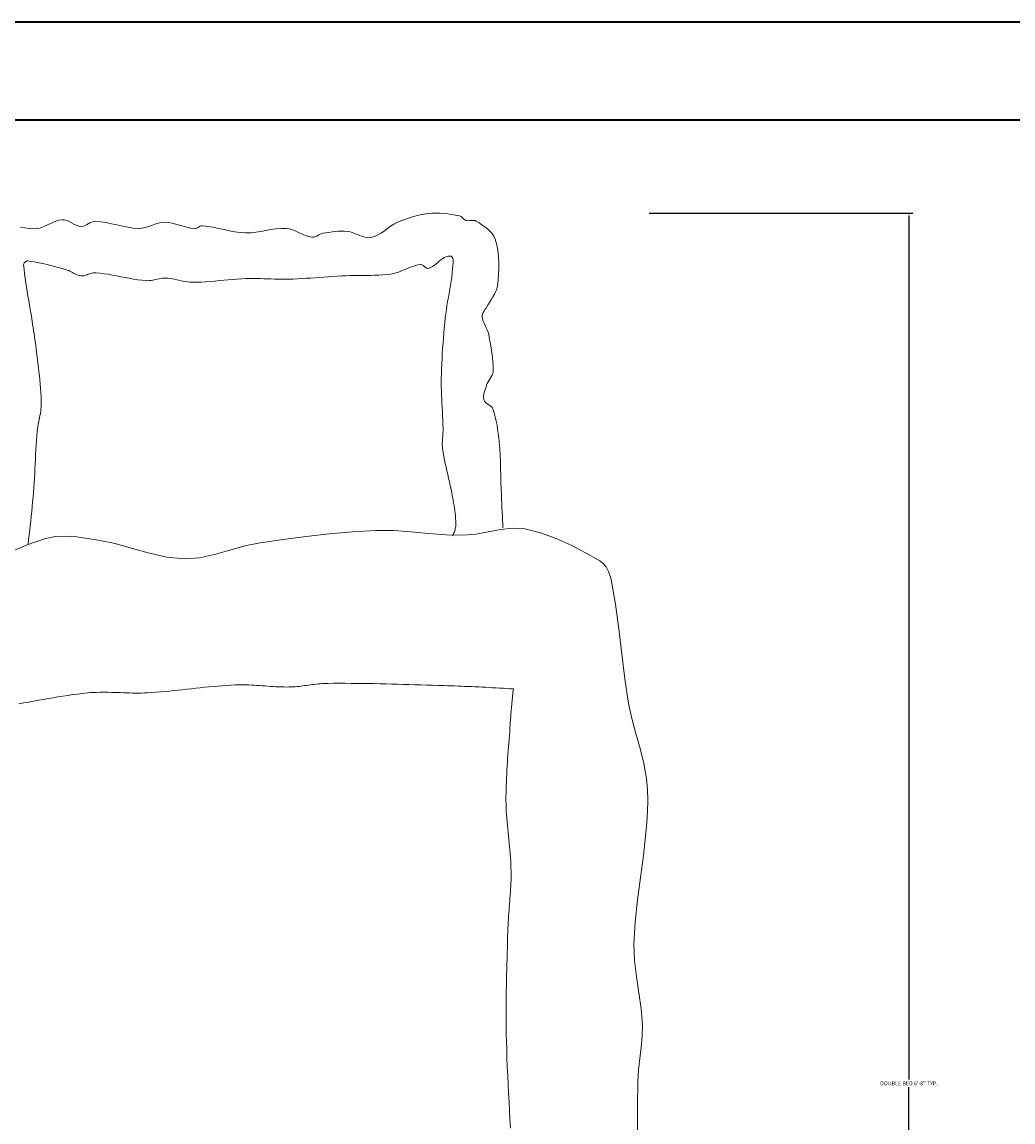
# Model space of a CAD drawing. Units: inches. Extents: x -36302355 to 648, y -221479757 to 75.
# Tile 27 of 37: x 220 to 265, y -218 to -167. Entities that reach past the tile are written whole.
import ezdxf

# ---------------------------------------------------------------- set-up
doc = ezdxf.new("R2010")
doc.units = ezdxf.units.IN
doc.header["$MEASUREMENT"] = 0
for name, color, linetype, lineweight in [('A-ANNO-DIMS', 2, 'Continuous', 18), ('A-FURN', 8, 'Continuous', 13), ('A-WALL', 7, 'Continuous', 35)]:
    doc.layers.add(name, color=color, linetype=linetype, lineweight=lineweight)
doc.styles.get("Standard").update_dxf_attribs({"font": 'arial.ttf'})
doc.dimstyles.get("Standard").update_dxf_attribs({"dimtxt": 0.18, "dimasz": 0.18, "dimexe": 0.18, "dimexo": 0.0625, "dimgap": 0.09, "dimtad": 0, "dimtih": 1, "dimtoh": 1, "dimdec": 0, "dimzin": 0, "dimdsep": 46, "dimlunit": 3, "dimtxsty": 'Standard', "dimcen": 0.09, "dimadec": 0, "dimazin": 0, "dimtfac": 1, "dimtdec": 0, "dimtofl": 0, "dimtmove": 0, "dimatfit": 3, "dimfxl": 1, "dimtolj": 1, "dimtzin": 0, "dimarcsym": 0})

# ---------------------------------------------------------------- blocks, each defined once
blk = doc.blocks.new('BED-DOUBLE')
for p, q in [((45.912, 79.943), (45.733, 79.9)), ((46.094, 79.977), (45.912, 79.943)), ((46.276, 80.001), (46.094, 79.977)), ((46.457, 80.015), (46.276, 80.001)), ((46.638, 80.019), (46.457, 80.015)), ((46.819, 80.013), (46.638, 80.019)), ((47.001, 80.001), (46.819, 80.013)), ((47.182, 79.981), (47.001, 80.001)), ((47.363, 79.957), (47.182, 79.981)), ((47.542, 79.928), (47.363, 79.957)), ((47.721, 79.897), (47.542, 79.928)), ((28.75, 79.461), (28.614, 79.399)), ((28.885, 79.529), (28.75, 79.461)), ((29.019, 79.595), (28.885, 79.529)), ((29.156, 79.653), (29.019, 79.595)), ((29.295, 79.695), (29.156, 79.653)), ((29.439, 79.716), (29.295, 79.695)), ((29.555, 79.707), (29.439, 79.716)), ((29.667, 79.676), (29.555, 79.707)), ((29.776, 79.63), (29.667, 79.676)), ((29.885, 79.575), (29.776, 79.63)), ((29.994, 79.518), (29.885, 79.575)), ((30.103, 79.467), (29.994, 79.518)), ((30.215, 79.429), (30.103, 79.467)), ((30.331, 79.412), (30.215, 79.429)), ((30.415, 79.419), (30.331, 79.412)), ((30.496, 79.445), (30.415, 79.419)), ((30.575, 79.483), (30.496, 79.445)), ((30.654, 79.527), (30.575, 79.483)), ((30.732, 79.571), (30.654, 79.527)), ((30.811, 79.61), (30.732, 79.571)), ((30.892, 79.636), (30.811, 79.61)), ((30.976, 79.644), (30.892, 79.636)), ((31.228, 79.624), (30.976, 79.644)), ((31.477, 79.585), (31.228, 79.624)), ((31.725, 79.534), (31.477, 79.585)), ((31.973, 79.478), (31.725, 79.534)), ((32.221, 79.421), (31.973, 79.478)), ((32.469, 79.372), (32.221, 79.421)), ((33.423, 79.406), (33.273, 79.362)), ((33.571, 79.458), (33.423, 79.406)), ((33.72, 79.51), (33.571, 79.458)), ((33.869, 79.555), (33.72, 79.51)), ((34.02, 79.587), (33.869, 79.555)), ((34.173, 79.598), (34.02, 79.587)), ((34.345, 79.587), (34.173, 79.598)), ((34.515, 79.557), (34.345, 79.587)), ((34.684, 79.516), (34.515, 79.557)), ((34.852, 79.467), (34.684, 79.516)), ((35.02, 79.416), (34.852, 79.467)), ((35.188, 79.369), (35.02, 79.416)), ((35.804, 79.42), (35.758, 79.398)), ((35.85, 79.435), (35.804, 79.42)), ((35.898, 79.439), (35.85, 79.435)), ((36.149, 79.41), (35.898, 79.439)), ((36.398, 79.368), (36.149, 79.41)), ((44.554, 79.421), (44.409, 79.317)), ((44.703, 79.516), (44.554, 79.421)), ((44.859, 79.595), (44.703, 79.516)), ((45.03, 79.665), (44.859, 79.595)), ((45.203, 79.731), (45.03, 79.665)), ((45.378, 79.793), (45.203, 79.731)), ((45.554, 79.85), (45.378, 79.793)), ((45.733, 79.9), (45.554, 79.85)), ((47.762, 79.883), (47.721, 79.897)), ((47.799, 79.86), (47.762, 79.883)), ((47.832, 79.831), (47.799, 79.86)), ((47.865, 79.797), (47.832, 79.831)), ((47.897, 79.763), (47.865, 79.797)), ((47.93, 79.732), (47.897, 79.763)), ((47.966, 79.705), (47.93, 79.732)), ((48.005, 79.687), (47.966, 79.705)), ((48.065, 79.675), (48.005, 79.687)), ((48.126, 79.673), (48.065, 79.675)), ((48.189, 79.677), (48.126, 79.673)), ((48.253, 79.684), (48.189, 79.677)), ((48.316, 79.688), (48.253, 79.684)), ((48.376, 79.687), (48.316, 79.688)), ((48.434, 79.676), (48.376, 79.687)), ((48.487, 79.652), (48.434, 79.676)), ((48.617, 79.57), (48.487, 79.652)), ((48.749, 79.484), (48.617, 79.57)), ((48.879, 79.394), (48.749, 79.484)), ((27.733, 79.348), (27.532, 79.381)), ((27.935, 79.319), (27.733, 79.348)), ((28.135, 79.305), (27.935, 79.319)), ((28.332, 79.316), (28.135, 79.305)), ((28.475, 79.348), (28.332, 79.316)), ((28.614, 79.399), (28.475, 79.348)), ((32.718, 79.336), (32.469, 79.372)), ((32.97, 79.321), (32.718, 79.336)), ((33.123, 79.331), (32.97, 79.321)), ((33.273, 79.362), (33.123, 79.331)), ((35.358, 79.33), (35.188, 79.369)), ((35.529, 79.305), (35.358, 79.33)), ((35.577, 79.308), (35.529, 79.305)), ((35.623, 79.323), (35.577, 79.308)), ((35.669, 79.345), (35.623, 79.323)), ((35.714, 79.371), (35.669, 79.345)), ((35.758, 79.398), (35.714, 79.371)), ((36.646, 79.318), (36.398, 79.368)), ((36.894, 79.264), (36.646, 79.318)), ((37.142, 79.212), (36.894, 79.264)), ((37.39, 79.167), (37.142, 79.212)), ((37.64, 79.133), (37.39, 79.167)), ((37.891, 79.115), (37.64, 79.133)), ((38.124, 79.119), (37.891, 79.115)), ((38.357, 79.144), (38.124, 79.119)), ((38.588, 79.18), (38.357, 79.144)), ((38.82, 79.223), (38.588, 79.18)), ((39.051, 79.265), (38.82, 79.223)), ((39.283, 79.299), (39.051, 79.265)), ((39.515, 79.318), (39.283, 79.299)), ((39.748, 79.315), (39.515, 79.318)), ((39.902, 79.292), (39.748, 79.315)), ((40.051, 79.248), (39.902, 79.292)), ((40.198, 79.189), (40.051, 79.248)), ((40.343, 79.122), (40.198, 79.189)), ((40.488, 79.055), (40.343, 79.122)), ((40.634, 78.992), (40.488, 79.055)), ((40.783, 78.942), (40.634, 78.992)), ((40.936, 78.91), (40.783, 78.942)), ((41.002, 78.91), (40.936, 78.91)), ((41.066, 78.924), (41.002, 78.91)), ((41.128, 78.95), (41.066, 78.924)), ((41.19, 78.981), (41.128, 78.95)), ((41.252, 79.016), (41.19, 78.981)), ((41.315, 79.048), (41.252, 79.016)), ((41.378, 79.075), (41.315, 79.048)), ((41.444, 79.093), (41.378, 79.075)), ((41.582, 79.116), (41.444, 79.093)), ((41.721, 79.137), (41.582, 79.116)), ((41.86, 79.157), (41.721, 79.137)), ((42, 79.173), (41.86, 79.157)), ((42.139, 79.184), (42, 79.173)), ((42.279, 79.19), (42.139, 79.184)), ((42.419, 79.19), (42.279, 79.19)), ((42.558, 79.182), (42.419, 79.19)), ((42.698, 79.158), (42.558, 79.182)), ((42.835, 79.114), (42.698, 79.158)), ((42.971, 79.06), (42.835, 79.114)), ((43.106, 79.003), (42.971, 79.06)), ((43.241, 78.95), (43.106, 79.003)), ((43.377, 78.91), (43.241, 78.95)), ((43.513, 78.89), (43.377, 78.91)), ((43.817, 78.944), (43.651, 78.898)), ((43.972, 79.016), (43.817, 78.944)), ((44.121, 79.107), (43.972, 79.016)), ((44.266, 79.21), (44.121, 79.107)), ((44.409, 79.317), (44.266, 79.21)), ((49.004, 79.298), (48.879, 79.394)), ((49.119, 79.194), (49.004, 79.298)), ((49.219, 79.081), (49.119, 79.194)), ((49.301, 78.957), (49.219, 79.081)), ((49.36, 78.82), (49.301, 78.957)), ((43.651, 78.898), (43.513, 78.89)), ((49.432, 78.561), (49.36, 78.82)), ((49.482, 78.296), (49.432, 78.561)), ((46.868, 77.87), (46.947, 77.928)), ((46.947, 77.928), (47.028, 77.978)), ((47.028, 77.978), (47.112, 78.016)), ((47.112, 78.016), (47.2, 78.041)), ((47.2, 78.041), (47.293, 78.049)), ((47.293, 78.049), (47.337, 78.04)), ((47.337, 78.04), (47.371, 78.018)), ((47.371, 78.018), (47.396, 77.983)), ((47.396, 77.983), (47.413, 77.939)), ((47.413, 77.939), (47.423, 77.887)), ((49.513, 78.027), (49.482, 78.296)), ((49.527, 77.755), (49.513, 78.027)), ((27.683, 77.649), (27.684, 77.671)), ((27.699, 77.441), (27.683, 77.649)), ((27.684, 77.671), (27.689, 77.693)), ((27.689, 77.693), (27.699, 77.715)), ((27.699, 77.715), (27.712, 77.735)), ((27.721, 77.234), (27.699, 77.441)), ((27.712, 77.735), (27.728, 77.755)), ((27.728, 77.755), (27.746, 77.773)), ((27.746, 77.773), (27.767, 77.789)), ((27.767, 77.789), (27.789, 77.803)), ((27.789, 77.803), (27.812, 77.813)), ((27.812, 77.813), (27.835, 77.821)), ((27.835, 77.821), (27.858, 77.824)), ((27.858, 77.824), (27.88, 77.824)), ((27.88, 77.824), (28.029, 77.804)), ((28.029, 77.804), (28.178, 77.781)), ((28.178, 77.781), (28.326, 77.754)), ((28.326, 77.754), (28.474, 77.723)), ((28.474, 77.723), (28.621, 77.691)), ((28.621, 77.691), (28.768, 77.655)), ((28.768, 77.655), (28.915, 77.618)), ((28.915, 77.618), (29.061, 77.58)), ((29.061, 77.58), (29.206, 77.54)), ((29.206, 77.54), (29.352, 77.499)), ((29.352, 77.499), (29.497, 77.458)), ((29.497, 77.458), (29.643, 77.417)), ((29.643, 77.417), (29.7, 77.398)), ((29.7, 77.398), (29.757, 77.376)), ((45.023, 77.35), (45.135, 77.394)), ((45.135, 77.394), (45.245, 77.439)), ((45.245, 77.439), (45.356, 77.485)), ((45.356, 77.485), (45.467, 77.529)), ((45.467, 77.529), (45.579, 77.57)), ((45.579, 77.57), (45.692, 77.607)), ((45.692, 77.607), (45.806, 77.636)), ((45.806, 77.636), (45.922, 77.659)), ((45.922, 77.659), (45.956, 77.659)), ((45.956, 77.659), (45.988, 77.65)), ((45.988, 77.65), (46.02, 77.634)), ((46.02, 77.634), (46.051, 77.613)), ((46.051, 77.613), (46.082, 77.589)), ((46.082, 77.589), (46.112, 77.564)), ((46.112, 77.564), (46.142, 77.538)), ((46.142, 77.538), (46.172, 77.515)), ((46.172, 77.515), (46.203, 77.496)), ((46.203, 77.496), (46.234, 77.483)), ((46.234, 77.483), (46.266, 77.478)), ((46.266, 77.478), (46.299, 77.482)), ((46.299, 77.482), (46.388, 77.515)), ((46.388, 77.515), (46.473, 77.56)), ((46.473, 77.56), (46.555, 77.615)), ((46.555, 77.615), (46.635, 77.677)), ((46.635, 77.677), (46.713, 77.741)), ((46.713, 77.741), (46.79, 77.807)), ((46.79, 77.807), (46.868, 77.87)), ((47.4, 77.462), (47.383, 77.273)), ((47.405, 77.515), (47.4, 77.462)), ((47.412, 77.574), (47.405, 77.515)), ((47.418, 77.637), (47.412, 77.574)), ((47.424, 77.701), (47.418, 77.637)), ((47.423, 77.887), (47.427, 77.828)), ((47.427, 77.766), (47.424, 77.701)), ((47.427, 77.828), (47.427, 77.766)), ((49.513, 77.208), (49.526, 77.481)), ((49.526, 77.481), (49.527, 77.755)), ((27.746, 77.027), (27.721, 77.234)), ((27.776, 76.821), (27.746, 77.027)), ((29.757, 77.376), (29.813, 77.349)), ((29.813, 77.349), (29.867, 77.321)), ((29.867, 77.321), (29.922, 77.292)), ((29.922, 77.292), (29.977, 77.263)), ((29.977, 77.263), (30.031, 77.234)), ((30.031, 77.234), (30.086, 77.207)), ((30.086, 77.207), (30.142, 77.184)), ((30.142, 77.184), (30.199, 77.164)), ((30.199, 77.164), (30.257, 77.148)), ((30.257, 77.148), (30.316, 77.139)), ((30.316, 77.139), (30.374, 77.137)), ((30.374, 77.137), (30.43, 77.142)), ((30.43, 77.142), (30.487, 77.153)), ((30.487, 77.153), (30.543, 77.169)), ((30.543, 77.169), (30.599, 77.187)), ((30.599, 77.187), (30.656, 77.207)), ((30.656, 77.207), (30.712, 77.227)), ((30.712, 77.227), (30.768, 77.246)), ((30.768, 77.246), (30.824, 77.261)), ((30.824, 77.261), (30.881, 77.273)), ((30.881, 77.273), (30.938, 77.28)), ((30.938, 77.28), (30.995, 77.28)), ((30.995, 77.28), (31.19, 77.261)), ((31.19, 77.261), (31.384, 77.237)), ((31.384, 77.237), (31.577, 77.207)), ((31.577, 77.207), (31.77, 77.173)), ((31.77, 77.173), (31.963, 77.137)), ((31.963, 77.137), (32.155, 77.099)), ((32.155, 77.099), (32.348, 77.062)), ((32.348, 77.062), (32.54, 77.025)), ((32.54, 77.025), (32.733, 76.991)), ((32.733, 76.991), (32.927, 76.961)), ((32.927, 76.961), (33.12, 76.936)), ((33.12, 76.936), (33.315, 76.917)), ((33.315, 76.917), (33.39, 76.915)), ((33.39, 76.915), (33.465, 76.919)), ((33.465, 76.919), (33.54, 76.927)), ((33.54, 76.927), (33.614, 76.939)), ((33.614, 76.939), (33.689, 76.954)), ((33.689, 76.954), (33.763, 76.97)), ((33.763, 76.97), (33.838, 76.986)), ((33.838, 76.986), (33.912, 77.002)), ((33.912, 77.002), (33.987, 77.015)), ((33.987, 77.015), (34.062, 77.026)), ((34.062, 77.026), (34.137, 77.032)), ((34.137, 77.032), (34.212, 77.032)), ((34.212, 77.032), (34.314, 77.026)), ((34.314, 77.026), (34.416, 77.014)), ((34.416, 77.014), (34.517, 76.997)), ((34.517, 76.997), (34.618, 76.978)), ((34.618, 76.978), (34.718, 76.956)), ((34.718, 76.956), (34.819, 76.934)), ((34.819, 76.934), (34.92, 76.912)), ((34.92, 76.912), (35.02, 76.891)), ((35.02, 76.891), (35.121, 76.873)), ((36.05, 76.866), (36.258, 76.881)), ((36.258, 76.881), (36.465, 76.899)), ((36.465, 76.899), (36.673, 76.918)), ((36.673, 76.918), (36.88, 76.938)), ((36.88, 76.938), (37.088, 76.957)), ((37.088, 76.957), (37.296, 76.976)), ((37.296, 76.976), (37.503, 76.992)), ((37.503, 76.992), (37.711, 77.005)), ((37.711, 77.005), (37.919, 77.014)), ((37.919, 77.014), (38.081, 77.017)), ((38.081, 77.017), (38.242, 77.017)), ((38.242, 77.017), (38.404, 77.015)), ((38.404, 77.015), (38.566, 77.011)), ((38.566, 77.011), (38.727, 77.006)), ((38.727, 77.006), (38.889, 77)), ((38.889, 77), (39.051, 76.993)), ((39.051, 76.993), (39.212, 76.988)), ((39.212, 76.988), (39.374, 76.984)), ((39.374, 76.984), (39.536, 76.981)), ((39.536, 76.981), (39.697, 76.981)), ((39.697, 76.981), (39.859, 76.984)), ((39.859, 76.984), (40.063, 76.991)), ((40.063, 76.991), (40.267, 77)), ((40.267, 77), (40.471, 77.011)), ((40.471, 77.011), (40.675, 77.024)), ((40.675, 77.024), (40.879, 77.038)), ((40.879, 77.038), (41.082, 77.053)), ((41.082, 77.053), (41.286, 77.068)), ((41.286, 77.068), (41.49, 77.083)), ((41.49, 77.083), (41.694, 77.098)), ((41.694, 77.098), (41.898, 77.112)), ((41.898, 77.112), (42.102, 77.125)), ((42.102, 77.125), (42.306, 77.136)), ((42.306, 77.136), (42.494, 77.144)), ((42.494, 77.144), (42.683, 77.148)), ((42.683, 77.148), (42.872, 77.151)), ((42.872, 77.151), (43.061, 77.152)), ((43.061, 77.152), (43.25, 77.152)), ((43.25, 77.152), (43.439, 77.153)), ((43.439, 77.153), (43.628, 77.156)), ((43.628, 77.156), (43.817, 77.161)), ((43.817, 77.161), (44.005, 77.169)), ((44.005, 77.169), (44.193, 77.181)), ((44.193, 77.181), (44.381, 77.199)), ((44.381, 77.199), (44.568, 77.222)), ((44.568, 77.222), (44.684, 77.244)), ((44.684, 77.244), (44.799, 77.273)), ((44.799, 77.273), (44.912, 77.309)), ((44.912, 77.309), (45.023, 77.35)), ((47.334, 76.896), (47.305, 76.708)), ((47.36, 77.084), (47.334, 76.896)), ((47.383, 77.273), (47.36, 77.084)), ((49.459, 76.667), (49.49, 76.936)), ((49.49, 76.936), (49.513, 77.208)), ((27.808, 76.615), (27.776, 76.821)), ((27.843, 76.41), (27.808, 76.615)), ((27.879, 76.204), (27.843, 76.41)), ((35.121, 76.873), (35.223, 76.858)), ((35.223, 76.858), (35.324, 76.848)), ((35.324, 76.848), (35.426, 76.845)), ((35.426, 76.845), (35.634, 76.847)), ((35.634, 76.847), (35.842, 76.854)), ((35.842, 76.854), (36.05, 76.866)), ((47.273, 76.52), (47.241, 76.333)), ((47.305, 76.708), (47.273, 76.52)), ((49.327, 76.292), (49.387, 76.412)), ((49.387, 76.412), (49.432, 76.537)), ((49.432, 76.537), (49.459, 76.667)), ((27.915, 75.999), (27.879, 76.204)), ((27.952, 75.793), (27.915, 75.999)), ((47.175, 75.958), (47.144, 75.77)), ((47.208, 76.145), (47.175, 75.958)), ((47.241, 76.333), (47.208, 76.145)), ((49.036, 75.827), (49.108, 75.944)), ((49.108, 75.944), (49.184, 76.059)), ((49.184, 76.059), (49.258, 76.175)), ((49.258, 76.175), (49.327, 76.292)), ((27.987, 75.588), (27.952, 75.793)), ((28.021, 75.382), (27.987, 75.588)), ((28.053, 75.176), (28.021, 75.382)), ((47.089, 75.394), (47.068, 75.205)), ((47.115, 75.582), (47.089, 75.394)), ((47.144, 75.77), (47.115, 75.582)), ((48.767, 75.329), (48.782, 75.386)), ((48.782, 75.386), (48.806, 75.441)), ((48.806, 75.441), (48.836, 75.495)), ((48.836, 75.495), (48.871, 75.549)), ((48.871, 75.549), (48.907, 75.602)), ((48.907, 75.602), (48.941, 75.655)), ((48.941, 75.655), (48.971, 75.709)), ((48.971, 75.709), (49.036, 75.827)), ((28.074, 75.036), (28.053, 75.176)), ((28.095, 74.896), (28.074, 75.036)), ((28.117, 74.755), (28.095, 74.896)), ((47.044, 74.972), (47.022, 74.739)), ((47.068, 75.205), (47.044, 74.972)), ((48.764, 75.269), (48.767, 75.329)), ((48.781, 75.161), (48.764, 75.269)), ((48.812, 75.056), (48.781, 75.161)), ((48.854, 74.954), (48.812, 75.056)), ((48.901, 74.853), (48.854, 74.954)), ((28.139, 74.615), (28.117, 74.755)), ((28.161, 74.475), (28.139, 74.615)), ((28.182, 74.335), (28.161, 74.475)), ((47.001, 74.505), (46.981, 74.272)), ((47.022, 74.739), (47.001, 74.505)), ((48.95, 74.751), (48.901, 74.853)), ((48.996, 74.649), (48.95, 74.751)), ((49.036, 74.546), (48.996, 74.649)), ((49.064, 74.439), (49.036, 74.546)), ((49.105, 74.229), (49.064, 74.439)), ((28.203, 74.194), (28.182, 74.335)), ((28.224, 74.054), (28.203, 74.194)), ((28.243, 73.914), (28.224, 74.054)), ((28.262, 73.773), (28.243, 73.914)), ((46.962, 74.038), (46.945, 73.805)), ((46.981, 74.272), (46.962, 74.038)), ((49.144, 74.017), (49.105, 74.229)), ((49.181, 73.805), (49.144, 74.017)), ((28.279, 73.632), (28.262, 73.773)), ((28.296, 73.491), (28.279, 73.632)), ((28.317, 73.302), (28.296, 73.491)), ((46.929, 73.571), (46.916, 73.337)), ((46.945, 73.805), (46.929, 73.571)), ((49.212, 73.592), (49.181, 73.805)), ((49.238, 73.379), (49.212, 73.592)), ((49.255, 73.166), (49.238, 73.379)), ((28.339, 73.113), (28.317, 73.302)), ((28.361, 72.924), (28.339, 73.113)), ((28.383, 72.734), (28.361, 72.924)), ((46.894, 72.869), (46.886, 72.635)), ((46.904, 73.103), (46.894, 72.869)), ((46.916, 73.337), (46.904, 73.103)), ((49.263, 72.952), (49.255, 73.166)), ((49.26, 72.738), (49.263, 72.952)), ((28.404, 72.545), (28.383, 72.734)), ((28.424, 72.356), (28.404, 72.545)), ((28.442, 72.166), (28.424, 72.356)), ((46.88, 72.401), (46.878, 72.212)), ((46.886, 72.635), (46.88, 72.401)), ((49.04, 72.269), (49.087, 72.345)), ((49.087, 72.345), (49.136, 72.42)), ((49.136, 72.42), (49.181, 72.496)), ((49.181, 72.496), (49.22, 72.573)), ((49.22, 72.573), (49.248, 72.654)), ((49.248, 72.654), (49.26, 72.738)), ((28.458, 71.976), (28.442, 72.166)), ((28.471, 71.786), (28.458, 71.976)), ((46.878, 72.212), (46.88, 72.024)), ((46.88, 72.024), (46.885, 71.835)), ((46.885, 71.835), (46.892, 71.647)), ((48.856, 71.777), (48.88, 71.861)), ((48.88, 71.861), (48.909, 71.945)), ((48.909, 71.945), (48.938, 72.028)), ((48.938, 72.028), (48.965, 72.11)), ((48.965, 72.11), (48.998, 72.191)), ((48.998, 72.191), (49.04, 72.269)), ((28.482, 71.596), (28.471, 71.786)), ((28.488, 71.406), (28.482, 71.596)), ((28.491, 71.216), (28.488, 71.406)), ((46.892, 71.647), (46.902, 71.458)), ((46.902, 71.458), (46.912, 71.27)), ((48.827, 71.607), (48.837, 71.692)), ((48.828, 71.523), (48.827, 71.607)), ((48.842, 71.44), (48.828, 71.523)), ((48.837, 71.692), (48.856, 71.777)), ((48.872, 71.375), (48.842, 71.44)), ((48.919, 71.32), (48.872, 71.375)), ((48.978, 71.271), (48.919, 71.32)), ((28.432, 70.709), (28.451, 70.81)), ((28.451, 70.81), (28.467, 70.911)), ((28.467, 70.911), (28.48, 71.012)), ((28.48, 71.012), (28.488, 71.114)), ((28.488, 71.114), (28.491, 71.216)), ((46.912, 71.27), (46.923, 71.081)), ((46.923, 71.081), (46.934, 70.893)), ((46.934, 70.893), (46.944, 70.704)), ((49.043, 71.226), (48.978, 71.271)), ((49.109, 71.182), (49.043, 71.226)), ((49.17, 71.134), (49.109, 71.182)), ((49.221, 71.08), (49.17, 71.134)), ((49.256, 71.016), (49.221, 71.08)), ((49.316, 70.833), (49.256, 71.016)), ((49.367, 70.648), (49.316, 70.833)), ((28.33, 70.205), (28.348, 70.306)), ((28.348, 70.306), (28.368, 70.407)), ((28.368, 70.407), (28.389, 70.508)), ((28.389, 70.508), (28.411, 70.608)), ((28.411, 70.608), (28.432, 70.709)), ((46.944, 70.704), (46.954, 70.516)), ((46.954, 70.516), (46.961, 70.327)), ((46.961, 70.327), (46.966, 70.138)), ((49.409, 70.46), (49.367, 70.648)), ((49.445, 70.27), (49.409, 70.46)), ((28.285, 69.785), (28.303, 70.002)), ((28.303, 70.002), (28.315, 70.104)), ((28.315, 70.104), (28.33, 70.205)), ((46.954, 69.822), (46.947, 69.743)), ((46.959, 69.901), (46.954, 69.822)), ((46.964, 69.98), (46.959, 69.901)), ((46.966, 70.059), (46.964, 69.98)), ((46.966, 70.138), (46.966, 70.059)), ((49.474, 70.079), (49.445, 70.27)), ((49.499, 69.887), (49.474, 70.079)), ((49.521, 69.695), (49.499, 69.887)), ((28.244, 69.133), (28.256, 69.35)), ((28.256, 69.35), (28.27, 69.568)), ((28.27, 69.568), (28.285, 69.785)), ((46.932, 69.506), (46.93, 69.427)), ((46.93, 69.427), (46.93, 69.349)), ((46.93, 69.349), (46.934, 69.27)), ((46.936, 69.585), (46.932, 69.506)), ((46.941, 69.664), (46.936, 69.585)), ((46.947, 69.743), (46.941, 69.664)), ((49.541, 69.503), (49.521, 69.695)), ((49.567, 69.196), (49.541, 69.503)), ((28.223, 68.697), (28.234, 68.915)), ((28.234, 68.915), (28.244, 69.133)), ((46.934, 69.27), (46.943, 69.192)), ((46.943, 69.192), (46.968, 69.02)), ((46.968, 69.02), (46.997, 68.85)), ((46.997, 68.85), (47.03, 68.679)), ((49.586, 68.889), (49.567, 69.196)), ((49.6, 68.581), (49.586, 68.889)), ((28.203, 68.262), (28.213, 68.48)), ((28.213, 68.48), (28.223, 68.697)), ((47.03, 68.679), (47.066, 68.51)), ((47.066, 68.51), (47.103, 68.34)), ((47.103, 68.34), (47.142, 68.171)), ((49.611, 68.273), (49.6, 68.581)), ((28.166, 67.61), (28.18, 67.827)), ((28.18, 67.827), (28.192, 68.045)), ((28.192, 68.045), (28.203, 68.262)), ((47.142, 68.171), (47.182, 68.002)), ((47.182, 68.002), (47.221, 67.833)), ((47.221, 67.833), (47.26, 67.664)), ((49.619, 67.964), (49.611, 68.273)), ((49.627, 67.656), (49.619, 67.964)), ((28.132, 67.176), (28.15, 67.392)), ((28.15, 67.392), (28.166, 67.61)), ((47.26, 67.664), (47.297, 67.495)), ((47.297, 67.495), (47.332, 67.325)), ((47.332, 67.325), (47.364, 67.155)), ((49.636, 67.348), (49.627, 67.656)), ((49.647, 67.04), (49.636, 67.348)), ((28.094, 66.742), (28.113, 66.959)), ((28.113, 66.959), (28.132, 67.176)), ((47.364, 67.155), (47.385, 67.039)), ((47.385, 67.039), (47.406, 66.924)), ((47.406, 66.924), (47.428, 66.809)), ((47.428, 66.809), (47.448, 66.693)), ((49.655, 66.854), (49.647, 67.04)), ((49.664, 66.668), (49.655, 66.854)), ((28.032, 66.093), (28.053, 66.309)), ((28.053, 66.309), (28.074, 66.526)), ((28.074, 66.526), (28.094, 66.742)), ((47.448, 66.693), (47.468, 66.577)), ((47.468, 66.577), (47.487, 66.462)), ((47.487, 66.462), (47.504, 66.346)), ((47.504, 66.346), (47.519, 66.23)), ((49.672, 66.482), (49.664, 66.668)), ((49.68, 66.296), (49.672, 66.482)), ((49.689, 66.11), (49.68, 66.296)), ((27.987, 65.66), (28.01, 65.876)), ((28.01, 65.876), (28.032, 66.093)), ((47.519, 66.23), (47.532, 66.113)), ((47.532, 66.113), (47.543, 65.997)), ((47.543, 65.997), (47.55, 65.88)), ((47.55, 65.88), (47.554, 65.763)), ((47.554, 65.763), (47.553, 65.713)), ((49.697, 65.924), (49.689, 66.11)), ((49.706, 65.738), (49.697, 65.924)), ((27.938, 65.228), (27.963, 65.444)), ((27.963, 65.444), (27.987, 65.66)), ((41.735, 65.273), (40.671, 65.153)), ((42.802, 65.366), (41.735, 65.273)), ((43.87, 65.425), (42.802, 65.366)), ((44.678, 65.422), (43.87, 65.425)), ((45.485, 65.369), (44.678, 65.422)), ((46.292, 65.296), (45.485, 65.369)), ((47.1, 65.235), (46.292, 65.296)), ((47.445, 65.274), (47.422, 65.229)), ((47.466, 65.32), (47.445, 65.274)), ((47.484, 65.367), (47.466, 65.32)), ((47.501, 65.415), (47.484, 65.367)), ((47.515, 65.464), (47.501, 65.415)), ((47.527, 65.513), (47.515, 65.464)), ((47.537, 65.563), (47.527, 65.513)), ((47.545, 65.613), (47.537, 65.563)), ((47.55, 65.663), (47.545, 65.613)), ((47.553, 65.713), (47.55, 65.663)), ((48.474, 65.264), (47.908, 65.214)), ((49.04, 65.369), (48.474, 65.264)), ((49.604, 65.477), (49.04, 65.369)), ((50.166, 65.538), (49.604, 65.477)), ((49.715, 65.552), (49.706, 65.738)), ((50.724, 65.499), (50.166, 65.538)), ((51.45, 65.318), (50.724, 65.499)), ((52.158, 65.065), (51.45, 65.318)), ((27.839, 64.768), (27.022, 64.416)), ((28.68, 65.056), (27.839, 64.768)), ((27.887, 64.796), (27.913, 65.012)), ((27.913, 65.012), (27.938, 65.228)), ((29.152, 65.148), (28.68, 65.056)), ((29.636, 65.165), (29.152, 65.148)), ((30.126, 65.13), (29.636, 65.165)), ((30.616, 65.064), (30.126, 65.13)), ((31.101, 64.99), (30.616, 65.064)), ((31.896, 64.828), (31.101, 64.99)), ((32.683, 64.608), (31.896, 64.828)), ((38.549, 64.862), (37.849, 64.716)), ((39.609, 65.014), (38.549, 64.862)), ((40.671, 65.153), (39.609, 65.014)), ((47.908, 65.214), (47.1, 65.235)), ((47.422, 65.229), (47.397, 65.186)), ((52.846, 64.755), (52.158, 65.065)), ((53.517, 64.405), (52.846, 64.755)), ((33.469, 64.384), (32.683, 64.608)), ((34.259, 64.206), (33.469, 64.384)), ((36.463, 64.326), (35.767, 64.177)), ((37.155, 64.522), (36.463, 64.326)), ((37.849, 64.716), (37.155, 64.522)), ((54.172, 64.032), (53.517, 64.405)), ((35.061, 64.125), (34.259, 64.206)), ((35.767, 64.177), (35.061, 64.125)), ((54.33, 63.91), (54.172, 64.032)), ((54.459, 63.752), (54.33, 63.91)), ((54.561, 63.57), (54.459, 63.752)), ((54.638, 63.375), (54.561, 63.57)), ((54.689, 63.176), (54.638, 63.375)), ((54.886, 62.042), (54.689, 63.176)), ((55.039, 60.9), (54.886, 62.042)), ((55.175, 59.755), (55.039, 60.9)), ((55.318, 58.611), (55.175, 59.755)), ((35.594, 58.175), (35.393, 58.153)), ((35.796, 58.197), (35.594, 58.175)), ((35.998, 58.218), (35.796, 58.197)), ((36.2, 58.239), (35.998, 58.218)), ((36.401, 58.258), (36.2, 58.239)), ((36.603, 58.276), (36.401, 58.258)), ((36.806, 58.292), (36.603, 58.276)), ((37.008, 58.306), (36.806, 58.292)), ((37.21, 58.318), (37.008, 58.306)), ((37.413, 58.327), (37.21, 58.318)), ((37.537, 58.331), (37.413, 58.327)), ((37.661, 58.333), (37.537, 58.331)), ((37.785, 58.332), (37.661, 58.333)), ((37.909, 58.329), (37.785, 58.332)), ((38.034, 58.325), (37.909, 58.329)), ((38.158, 58.319), (38.034, 58.325)), ((38.282, 58.313), (38.158, 58.319)), ((38.406, 58.305), (38.282, 58.313)), ((38.53, 58.296), (38.406, 58.305)), ((38.654, 58.288), (38.53, 58.296)), ((38.779, 58.279), (38.654, 58.288)), ((38.903, 58.27), (38.779, 58.279)), ((39.027, 58.261), (38.903, 58.27)), ((39.151, 58.253), (39.027, 58.261)), ((39.275, 58.246), (39.151, 58.253)), ((39.4, 58.241), (39.275, 58.246)), ((39.524, 58.236), (39.4, 58.241)), ((39.648, 58.233), (39.524, 58.236)), ((39.772, 58.232), (39.648, 58.233)), ((39.896, 58.233), (39.772, 58.232)), ((39.985, 58.235), (39.896, 58.233)), ((40.073, 58.24), (39.985, 58.235)), ((40.162, 58.246), (40.073, 58.24)), ((40.25, 58.254), (40.162, 58.246)), ((40.338, 58.262), (40.25, 58.254)), ((40.426, 58.272), (40.338, 58.262)), ((40.514, 58.283), (40.426, 58.272)), ((40.603, 58.294), (40.514, 58.283)), ((40.691, 58.306), (40.603, 58.294)), ((40.779, 58.318), (40.691, 58.306)), ((40.867, 58.33), (40.779, 58.318)), ((40.955, 58.342), (40.867, 58.33)), ((41.043, 58.353), (40.955, 58.342)), ((41.131, 58.363), (41.043, 58.353)), ((41.219, 58.373), (41.131, 58.363)), ((41.307, 58.381), (41.219, 58.373)), ((41.395, 58.389), (41.307, 58.381)), ((41.484, 58.394), (41.395, 58.389)), ((41.572, 58.398), (41.484, 58.394)), ((41.661, 58.4), (41.572, 58.398)), ((41.928, 58.402), (41.661, 58.4)), ((42.196, 58.402), (41.928, 58.402)), ((42.464, 58.402), (42.196, 58.402)), ((42.731, 58.401), (42.464, 58.402)), ((42.999, 58.398), (42.731, 58.401)), ((43.267, 58.395), (42.999, 58.398)), ((43.535, 58.391), (43.267, 58.395)), ((43.802, 58.386), (43.535, 58.391)), ((44.07, 58.381), (43.802, 58.386)), ((44.338, 58.375), (44.07, 58.381)), ((44.605, 58.368), (44.338, 58.375)), ((44.873, 58.362), (44.605, 58.368)), ((45.141, 58.354), (44.873, 58.362)), ((45.408, 58.346), (45.141, 58.354)), ((45.676, 58.339), (45.408, 58.346)), ((45.944, 58.33), (45.676, 58.339)), ((46.211, 58.322), (45.944, 58.33)), ((46.479, 58.314), (46.211, 58.322)), ((46.746, 58.306), (46.479, 58.314)), ((47.014, 58.298), (46.746, 58.306)), ((47.173, 58.293), (47.014, 58.298)), ((47.333, 58.287), (47.173, 58.293)), ((47.492, 58.282), (47.333, 58.287)), ((47.651, 58.276), (47.492, 58.282)), ((47.81, 58.27), (47.651, 58.276)), ((47.97, 58.263), (47.81, 58.27)), ((48.129, 58.257), (47.97, 58.263)), ((48.288, 58.25), (48.129, 58.257)), ((48.447, 58.242), (48.288, 58.25)), ((48.606, 58.235), (48.447, 58.242)), ((48.766, 58.227), (48.606, 58.235)), ((48.925, 58.219), (48.766, 58.227)), ((49.084, 58.21), (48.925, 58.219)), ((49.243, 58.201), (49.084, 58.21)), ((49.402, 58.192), (49.243, 58.201)), ((49.561, 58.183), (49.402, 58.192)), ((49.72, 58.173), (49.561, 58.183)), ((49.879, 58.163), (49.72, 58.173)), ((55.495, 57.473), (55.318, 58.611)), ((28.588, 57.662), (28.364, 57.622)), ((28.812, 57.702), (28.588, 57.662)), ((29.036, 57.741), (28.812, 57.702)), ((29.261, 57.778), (29.036, 57.741)), ((29.485, 57.815), (29.261, 57.778)), ((29.71, 57.849), (29.485, 57.815)), ((29.935, 57.881), (29.71, 57.849)), ((30.161, 57.91), (29.935, 57.881)), ((30.386, 57.937), (30.161, 57.91)), ((30.613, 57.96), (30.386, 57.937)), ((30.75, 57.972), (30.613, 57.96)), ((30.888, 57.98), (30.75, 57.972)), ((31.026, 57.986), (30.888, 57.98)), ((31.163, 57.989), (31.026, 57.986)), ((31.301, 57.991), (31.163, 57.989)), ((31.439, 57.99), (31.301, 57.991)), ((31.577, 57.988), (31.439, 57.99)), ((31.716, 57.985), (31.577, 57.988)), ((31.854, 57.981), (31.716, 57.985)), ((31.992, 57.977), (31.854, 57.981)), ((32.13, 57.972), (31.992, 57.977)), ((32.268, 57.967), (32.13, 57.972)), ((32.407, 57.963), (32.268, 57.967)), ((32.545, 57.959), (32.407, 57.963)), ((32.683, 57.956), (32.545, 57.959)), ((32.821, 57.954), (32.683, 57.956)), ((32.959, 57.954), (32.821, 57.954)), ((33.097, 57.956), (32.959, 57.954)), ((33.235, 57.959), (33.097, 57.956)), ((33.373, 57.965), (33.235, 57.959)), ((33.576, 57.978), (33.373, 57.965)), ((33.778, 57.992), (33.576, 57.978)), ((33.98, 58.008), (33.778, 57.992)), ((34.182, 58.026), (33.98, 58.008)), ((34.384, 58.045), (34.182, 58.026)), ((34.586, 58.065), (34.384, 58.045)), ((34.788, 58.087), (34.586, 58.065)), ((34.989, 58.108), (34.788, 58.087)), ((35.191, 58.131), (34.989, 58.108)), ((35.393, 58.153), (35.191, 58.131)), ((50.038, 58.153), (49.879, 58.163)), ((50.197, 58.142), (50.038, 58.153)), ((50.137, 57.577), (50.145, 57.658)), ((50.145, 57.658), (50.153, 57.739)), ((50.153, 57.739), (50.162, 57.82)), ((50.162, 57.82), (50.17, 57.9)), ((50.17, 57.9), (50.179, 57.981)), ((50.179, 57.981), (50.188, 58.062)), ((50.188, 58.062), (50.197, 58.142)), ((27.691, 57.503), (27.467, 57.465)), ((27.916, 57.542), (27.691, 57.503)), ((28.14, 57.582), (27.916, 57.542)), ((28.364, 57.622), (28.14, 57.582)), ((50.093, 57.092), (50.1, 57.173)), ((50.1, 57.173), (50.107, 57.254)), ((50.107, 57.254), (50.114, 57.335)), ((50.114, 57.335), (50.122, 57.416)), ((50.122, 57.416), (50.129, 57.497)), ((50.129, 57.497), (50.137, 57.577)), ((55.646, 56.779), (55.495, 57.473)), ((50.056, 56.607), (50.062, 56.688)), ((50.062, 56.688), (50.068, 56.769)), ((50.068, 56.769), (50.074, 56.85)), ((50.074, 56.85), (50.08, 56.931)), ((50.08, 56.931), (50.086, 57.012)), ((50.086, 57.012), (50.093, 57.092)), ((55.831, 56.091), (55.646, 56.779)), ((50.013, 56), (50.026, 56.175)), ((50.026, 56.175), (50.039, 56.35)), ((50.039, 56.35), (50.051, 56.526)), ((50.051, 56.526), (50.056, 56.607)), ((49.973, 55.474), (49.987, 55.649)), ((49.987, 55.649), (50, 55.824)), ((50, 55.824), (50.013, 56)), ((56.024, 55.406), (55.831, 56.091)), ((49.947, 55.123), (49.96, 55.298)), ((49.96, 55.298), (49.973, 55.474)), ((56.197, 54.717), (56.024, 55.406)), ((49.91, 54.596), (49.922, 54.772)), ((49.922, 54.772), (49.934, 54.947)), ((49.934, 54.947), (49.947, 55.123)), ((56.323, 54.019), (56.197, 54.717)), ((49.881, 54.07), (49.89, 54.245)), ((49.89, 54.245), (49.9, 54.421)), ((49.9, 54.421), (49.91, 54.596)), ((49.862, 53.543), (49.867, 53.719)), ((49.867, 53.719), (49.873, 53.894)), ((49.873, 53.894), (49.881, 54.07)), ((56.369, 53.519), (56.323, 54.019)), ((49.857, 53.192), (49.859, 53.367)), ((49.857, 53.016), (49.857, 53.192)), ((49.859, 53.367), (49.862, 53.543)), ((56.379, 53.016), (56.369, 53.519)), ((49.859, 52.853), (49.857, 53.016)), ((49.865, 52.69), (49.859, 52.853)), ((49.872, 52.527), (49.865, 52.69)), ((56.363, 52.512), (56.379, 53.016)), ((49.882, 52.365), (49.872, 52.527)), ((49.894, 52.202), (49.882, 52.365)), ((49.907, 52.04), (49.894, 52.202)), ((56.33, 52.008), (56.363, 52.512)), ((49.922, 51.877), (49.907, 52.04)), ((49.938, 51.715), (49.922, 51.877)), ((49.954, 51.553), (49.938, 51.715)), ((56.292, 51.505), (56.33, 52.008)), ((49.971, 51.39), (49.954, 51.553)), ((49.988, 51.228), (49.971, 51.39)), ((50.004, 51.065), (49.988, 51.228)), ((56.186, 50.484), (56.292, 51.505)), ((50.02, 50.903), (50.004, 51.065)), ((50.035, 50.741), (50.02, 50.903)), ((50.049, 50.578), (50.035, 50.741)), ((50.062, 50.416), (50.049, 50.578)), ((50.072, 50.253), (50.062, 50.416)), ((50.081, 50.09), (50.072, 50.253)), ((50.087, 49.927), (50.081, 50.09)), ((56.047, 49.466), (56.186, 50.484)), ((50.091, 49.764), (50.087, 49.927)), ((50.092, 49.626), (50.091, 49.764)), ((50.091, 49.488), (50.092, 49.626)), ((50.069, 48.935), (50.077, 49.073)), ((50.077, 49.073), (50.083, 49.211)), ((50.083, 49.211), (50.088, 49.349)), ((50.088, 49.349), (50.091, 49.488)), ((55.905, 48.448), (56.047, 49.466)), ((50.041, 48.52), (50.051, 48.658)), ((50.051, 48.658), (50.061, 48.797)), ((50.061, 48.797), (50.069, 48.935)), ((49.998, 47.968), (50.009, 48.106)), ((50.009, 48.106), (50.02, 48.244)), ((50.02, 48.244), (50.031, 48.382)), ((50.031, 48.382), (50.041, 48.52)), ((55.79, 47.428), (55.905, 48.448)), ((49.959, 47.415), (49.968, 47.553)), ((49.968, 47.553), (49.977, 47.691)), ((49.977, 47.691), (49.987, 47.83)), ((49.987, 47.83), (49.998, 47.968)), ((49.941, 47), (49.946, 47.138)), ((49.946, 47.138), (49.952, 47.277)), ((49.952, 47.277), (49.959, 47.415)), ((55.733, 46.404), (55.79, 47.428)), ((49.927, 46.497), (49.934, 46.749)), ((49.934, 46.749), (49.941, 47)), ((49.913, 45.995), (49.92, 46.246)), ((49.92, 46.246), (49.927, 46.497)), ((55.763, 45.66), (55.733, 46.404)), ((49.899, 45.492), (49.906, 45.743)), ((49.906, 45.743), (49.913, 45.995)), ((55.854, 44.918), (55.763, 45.66)), ((49.887, 44.989), (49.893, 45.241)), ((49.893, 45.241), (49.899, 45.492)), ((49.876, 44.487), (49.881, 44.738)), ((49.881, 44.738), (49.887, 44.989)), ((55.971, 44.178), (55.854, 44.918)), ((49.868, 43.984), (49.872, 44.235)), ((49.872, 44.235), (49.876, 44.487)), ((56.076, 43.436), (55.971, 44.178)), ((49.864, 43.481), (49.866, 43.733)), ((49.866, 43.733), (49.868, 43.984)), ((49.863, 43.23), (49.864, 43.481)), ((49.863, 42.979), (49.863, 43.23)), ((56.134, 42.692), (56.076, 43.436)), ((49.865, 42.727), (49.863, 42.979)), ((49.868, 42.476), (49.865, 42.727)), ((56.124, 42.175), (56.134, 42.692)), ((49.872, 42.225), (49.868, 42.476)), ((49.878, 41.973), (49.872, 42.225)), ((56.078, 41.659), (56.124, 42.175)), ((49.889, 41.571), (49.878, 41.973)), ((49.903, 41.169), (49.889, 41.571)), ((56.015, 41.144), (56.078, 41.659)), ((49.918, 40.767), (49.903, 41.169)), ((55.955, 40.628), (56.015, 41.144)), ((49.935, 40.364), (49.918, 40.767)), ((55.918, 40.112), (55.955, 40.628)), ((49.954, 39.962), (49.935, 40.364)), ((49.974, 39.56), (49.954, 39.962)), ((55.898, 38.895), (55.918, 40.112)), ((49.996, 39.159), (49.974, 39.56)), ((50.018, 38.757), (49.996, 39.159)), ((50.04, 38.355), (50.018, 38.757)), ((55.907, 37.677), (55.898, 38.895)), ((50.064, 37.953), (50.04, 38.355))]:
    blk.add_line(p, q)
blk = doc.blocks.new('*D37')
at = {"layer": 'A-ANNO-DIMS', "color": 0, "lineweight": -2, "transparency": 16777216}
for p, q in [((248.653, -175.809), (260.774, -175.809)), ((260.594, -175.989), (260.594, -215.635)), ((260.594, -255.648), (260.594, -216.001)), ((248.653, -255.828), (260.774, -255.828))]:
    blk.add_line(p, q, dxfattribs=at)
at = {"layer": 'A-ANNO-DIMS', "color": 0, "transparency": 16777216}
for points in [[(260.564, -175.989), (260.624, -175.989), (260.594, -175.809)], [(260.564, -255.648), (260.624, -255.648), (260.594, -255.828)]]:
    blk.add_solid(points, dxfattribs=at)
at = {"layer": 'Defpoints', "color": 0, "transparency": 16777216}
for p in [(248.591, -175.809), (260.594, -175.809), (248.591, -255.828)]:
    blk.add_point(p, dxfattribs=at)
at = {"layer": 'A-ANNO-DIMS', "color": 0, "transparency": 16777216, "insert": (260.594, -215.818), "char_height": 0.18, "attachment_point": 5}
blk.add_mtext('\\A1;DOUBLE BED 6\'-8" TYP.', dxfattribs=at)

msp = doc.modelspace()

# ---------------------------------------------------------------- linework, layer by layer
at = {"layer": 'A-WALL'}
for p, q in [((145.197, -167.019), (323.197, -167.019)), ((154.197, -171.519), (314.197, -171.519))]:
    msp.add_line(p, q, dxfattribs=at)

# ---------------------------------------------------------------- block references
at = {"layer": 'A-FURN'}
msp.add_blockref('BED-DOUBLE', (192.212, -255.828), dxfattribs=at)

# ---------------------------------------------------------------- dimensions: what is measured, and where the dimension line sits
at = {"layer": 'A-ANNO-DIMS'}
dim = msp.add_linear_dim(base=(260.594, -175.809), p1=(248.591, -255.828), p2=(248.591, -175.809), angle=90, text='DOUBLE BED <> TYP.', dimstyle='Standard', override={"dimdec": 1, "dimlfac": 1, "dimrnd": 0, "dimzin": 1, "dimdsep": 46, "dimlunit": 4, "dimfrac": 2}, dxfattribs=at)
dim.commit()
dim.dimension.update_dxf_attribs({"geometry": '*D37', "text_midpoint": (260.594, -215.818)})

doc.saveas('drawing.dxf')
